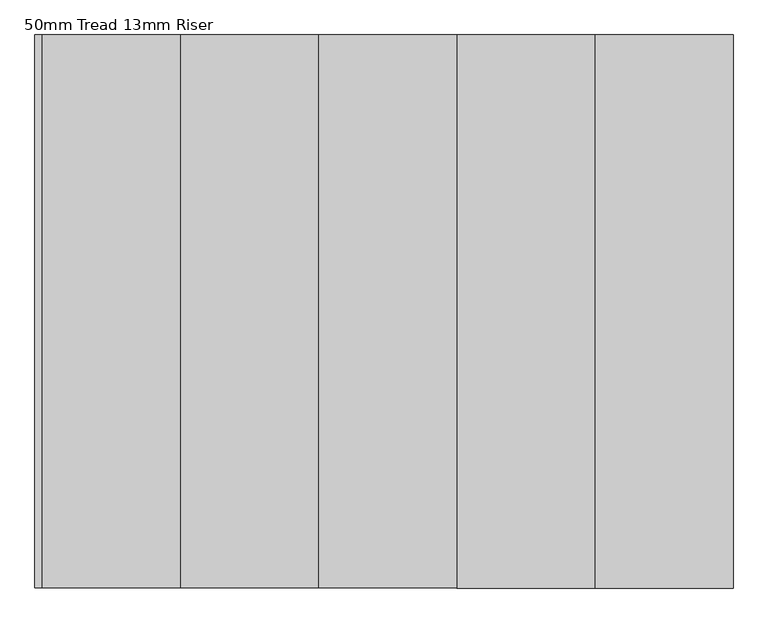
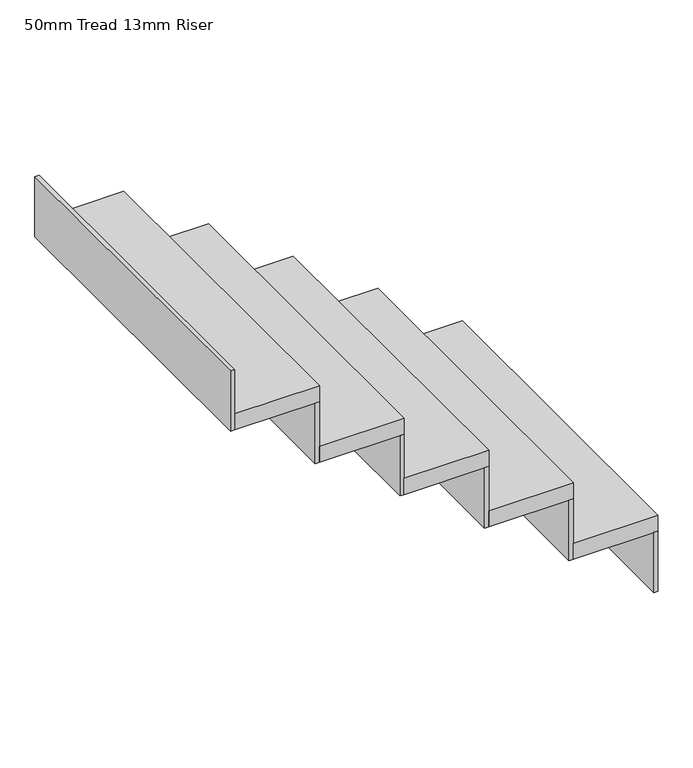
"""IFC4 building model written with IfcOpenShell, lengths in millimetres: stair flight geometry, 50mm Tread 13mm Riser."""

from ifc_helpers import new_model, si_unit, frame, origin, place, context, project, spatial, polyline, outline, extrude, source, transform, mapped, element, save


def stair_flight_50mm_tread_13mm_riser_70c7a40c(model_context):
    return source(origin(), model_context, "Body", "SweptSolid", [
        extrude(outline(polyline([(-10480.6794909, -3251.1360696), (-10468.1794909, -3251.1360696), (-10468.1794909, -4251.1618509), (-10480.6794909, -4251.1618509), (-10480.6794909, -3251.1360696)])), frame((0.0, 0.0, 5221.2470588), z_axis=(0.0, 0.0, 1.0), x_axis=(1.0, 0.0, 0.0)), (0.0, 0.0, 1.0), 188.2588235),
        extrude(outline(polyline([(-10718.1794909, -4251.1618509), (-10718.1794909, -3251.1360696), (-10468.1794909, -3251.1360696), (-10468.1794909, -4251.1618509), (-10718.1794909, -4251.1618509)])), frame((0.0, 0.0, 5409.5058824), z_axis=(0.0, 0.0, 1.0), x_axis=(1.0, 0.0, 0.0)), (0.0, 0.0, 1.0), 50.0),
        extrude(outline(polyline([(-10730.6794909, -3251.1360696), (-10718.1794909, -3251.1360696), (-10718.1794909, -4251.1618509), (-10730.6794909, -4251.1618509), (-10730.6794909, -3251.1360696)])), frame((0.0, 0.0, 5409.5058824), z_axis=(0.0, 0.0, 1.0), x_axis=(1.0, 0.0, 0.0)), (0.0, 0.0, 1.0), 188.2588235),
        extrude(outline(polyline([(-10968.1794909, -4251.1618509), (-10968.1794909, -3251.1360696), (-10718.1794909, -3251.1360696), (-10718.1794909, -4251.1618509), (-10968.1794909, -4251.1618509)])), frame((0.0, 0.0, 5597.7647059), z_axis=(0.0, 0.0, 1.0), x_axis=(1.0, 0.0, 0.0)), (0.0, 0.0, 1.0), 50.0),
        extrude(outline(polyline([(-10980.6794909, -3251.1360696), (-10968.1794909, -3251.1360696), (-10968.1794909, -4251.1618509), (-10980.6794909, -4251.1618509), (-10980.6794909, -3251.1360696)])), frame((0.0, 0.0, 5597.7647059), z_axis=(0.0, 0.0, 1.0), x_axis=(1.0, 0.0, 0.0)), (0.0, 0.0, 1.0), 188.2588235),
        extrude(outline(polyline([(-11218.1794909, -4251.1618509), (-11218.1794909, -3251.1360696), (-10968.1794909, -3251.1360696), (-10968.1794909, -4251.1618509), (-11218.1794909, -4251.1618509)])), frame((0.0, 0.0, 5786.0235294), z_axis=(0.0, 0.0, 1.0), x_axis=(1.0, 0.0, 0.0)), (0.0, 0.0, 1.0), 50.0),
        extrude(outline(polyline([(-11230.6794909, -3251.1360696), (-11218.1794909, -3251.1360696), (-11218.1794909, -4251.1618509), (-11230.6794909, -4251.1618509), (-11230.6794909, -3251.1360696)])), frame((0.0, 0.0, 5786.0235294), z_axis=(0.0, 0.0, 1.0), x_axis=(1.0, 0.0, 0.0)), (0.0, 0.0, 1.0), 188.2588235),
        extrude(outline(polyline([(-11468.1794909, -4251.1618509), (-11468.1794909, -3251.1360696), (-11218.1794909, -3251.1360696), (-11218.1794909, -4251.1618509), (-11468.1794909, -4251.1618509)])), frame((0.0, 0.0, 5974.2823529), z_axis=(0.0, 0.0, 1.0), x_axis=(1.0, 0.0, 0.0)), (0.0, 0.0, 1.0), 50.0),
        extrude(outline(polyline([(-11480.6794909, -3251.1360696), (-11468.1794909, -3251.1360696), (-11468.1794909, -4251.1618509), (-11480.6794909, -4251.1618509), (-11480.6794909, -3251.1360696)])), frame((0.0, 0.0, 5974.2823529), z_axis=(0.0, 0.0, 1.0), x_axis=(1.0, 0.0, 0.0)), (0.0, 0.0, 1.0), 188.2588235),
        extrude(outline(polyline([(-11730.6794909, -3251.1360696), (-11718.1794909, -3251.1360696), (-11718.1794909, -4251.1618509), (-11730.6794909, -4251.1618509), (-11730.6794909, -3251.1360696)])), frame((0.0, 0.0, 6162.5411765), z_axis=(0.0, 0.0, 1.0), x_axis=(1.0, 0.0, 0.0)), (0.0, 0.0, 1.0), 188.2588235),
        extrude(outline(polyline([(-11718.1794909, -4251.1618509), (-11718.1794909, -3251.1360696), (-11468.1794909, -3251.1360696), (-11468.1794909, -4251.1618509), (-11718.1794909, -4251.1618509)])), frame((0.0, 0.0, 6162.5411765), z_axis=(0.0, 0.0, 1.0), x_axis=(1.0, 0.0, 0.0)), (0.0, 0.0, 1.0), 50.0),
    ])


if __name__ == "__main__":
    model = new_model("IFC4")
    model_context = context("Model", 3, world=origin())
    ifc_project = project(units=[si_unit("LENGTHUNIT", "METRE", prefix="MILLI")], contexts=[model_context])
    site = spatial("IfcSite", under=ifc_project)
    building = spatial("IfcBuilding", under=site)
    placement = place(None, origin())
    stair_flight_50mm_tread_13mm_riser_shape = stair_flight_50mm_tread_13mm_riser_70c7a40c(model_context)
    element("IfcStairFlight", 1, ObjectType="50mm Tread 13mm Riser", at=placement, inside=building, context=model_context, shape_type="MappedRepresentation", body=[
        mapped(stair_flight_50mm_tread_13mm_riser_shape, transform((0.0, 0.0, 0.0), x_axis=(1.0, 0.0, 0.0), y_axis=(0.0, 1.0, 0.0), z_axis=(0.0, 0.0, 1.0))),
    ])
    save(model, "model.ifc")
